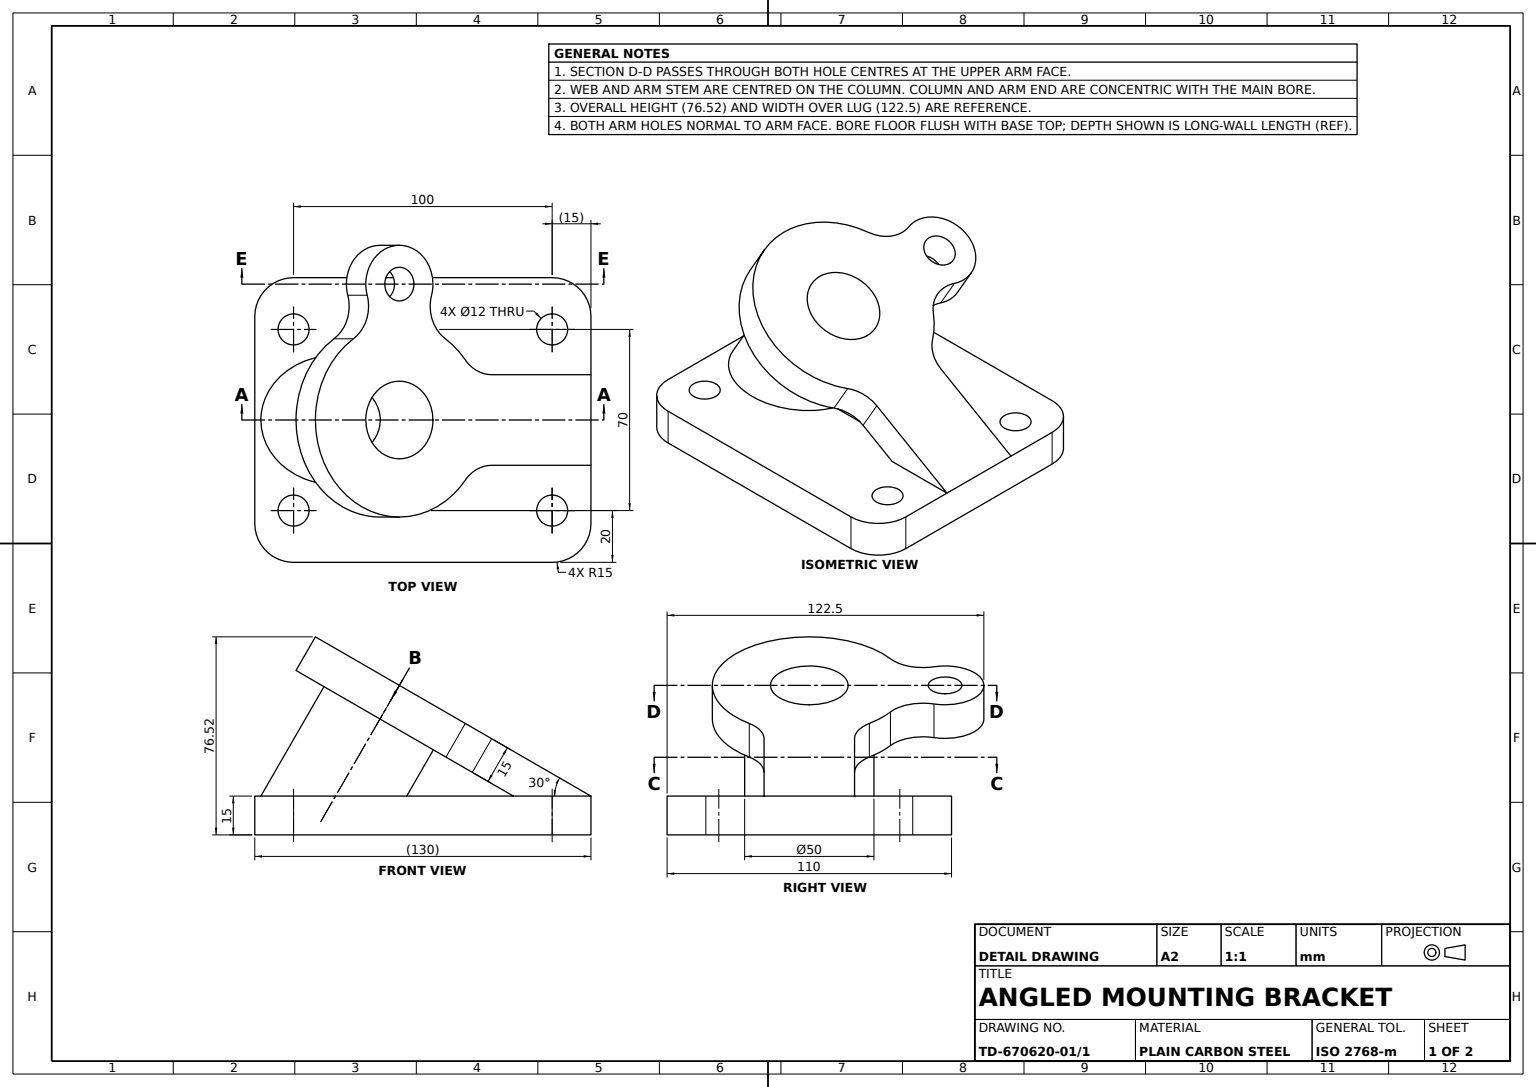
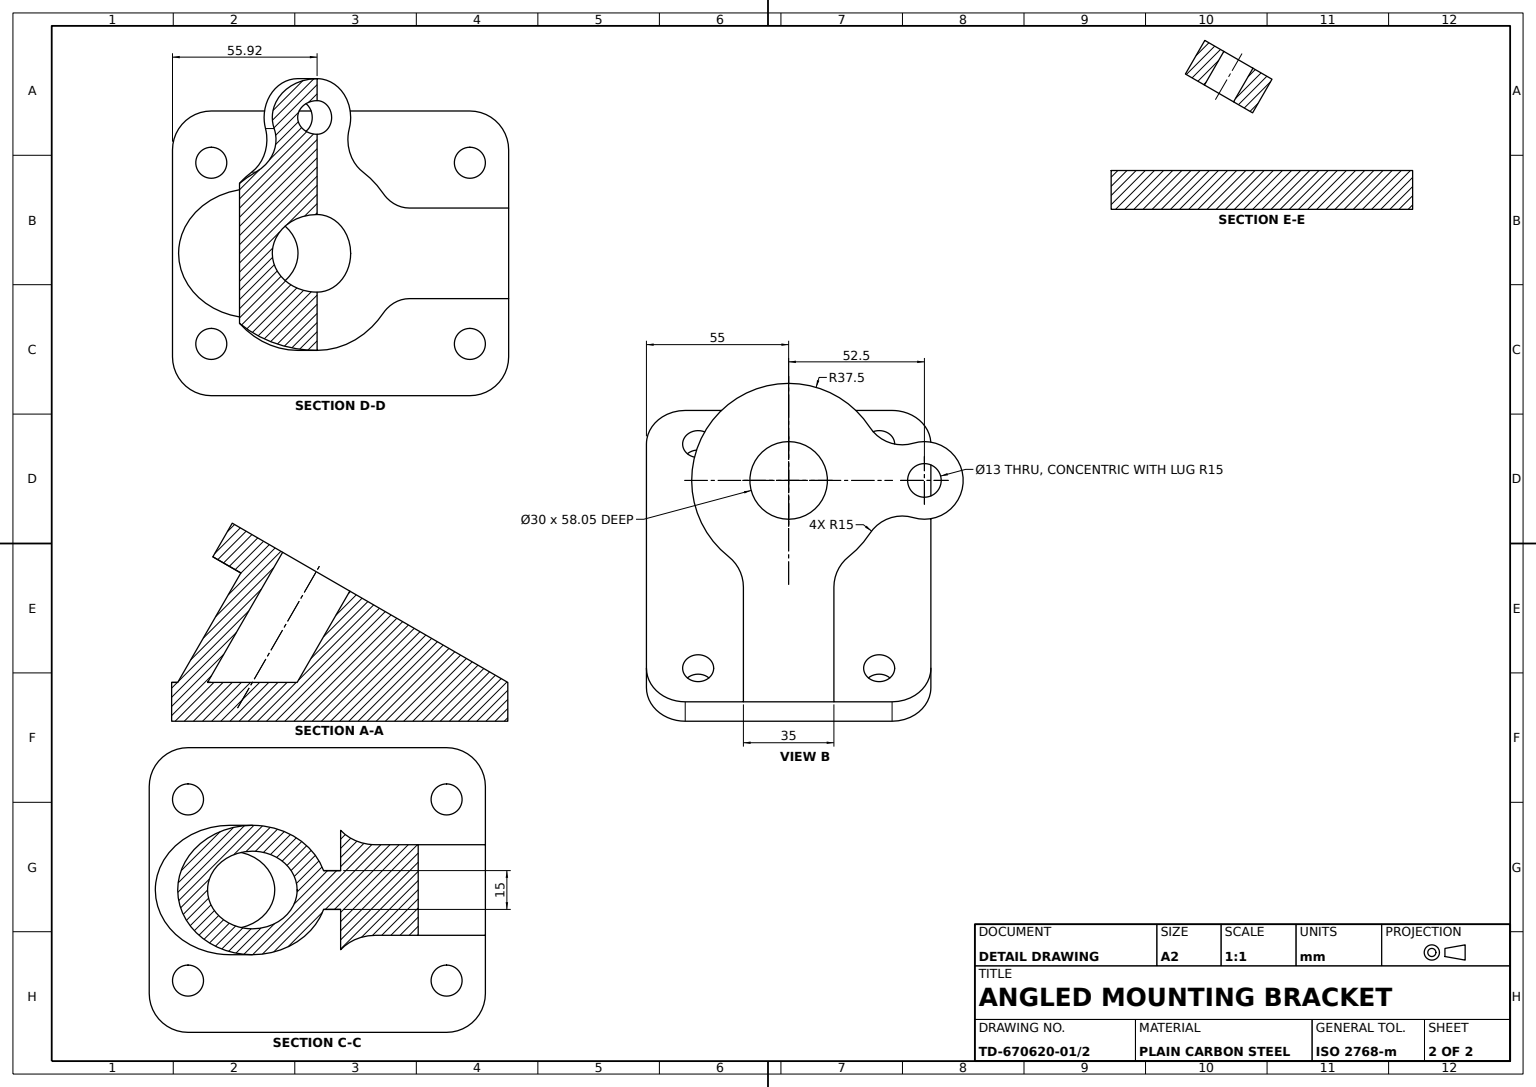
SolidWorks part; units mm, degrees
material "Plain Carbon Steel"
ref_plane "Front Plane" through (0, 0, 0) normal (0, 0, 1) x (1, 0, 0)
ref_plane "Top Plane" through (0, 0, 0) normal (0, 1, 0) x (1, 0, 0)
ref_plane "Right Plane" through (0, 0, 0) normal (1, 0, 0) x (0, 0, -1)
sketch "Base Plate Sketch" plane through (0, 0, 0) normal (0, 1, 0) x (1, 0, 0)
  line L0 (0, 119.1376) -> (0, -127.5955) construction
  line L1 (-50, 55) -> (50, 55)
  line L2 (-65, 40) -> (-65, -40)
  line L3 (-50, -55) -> (50, -55)
  line L4 (65, 40) -> (65, -40)
  line L5 (-65, 55) -> (65, -55) construction
  line L6 (-65, -55) -> (65, 55) construction
  line L7 (107.3268, 0) -> (-125.8206, 0) construction
  circle A0 centre (-50, 35) radius 6
  circle A1 centre (-50, -35) radius 6
  circle A2 centre (50, -35) radius 6
  circle A3 centre (50, 35) radius 6
  arc A4 (50, -55) -> (65, -40) centre (50, -40) ccw
  arc A5 (-65, -40) -> (-50, -55) centre (-50, -40) ccw
  arc A6 (-50, 55) -> (-65, 40) centre (-50, 40) ccw
  arc A7 (50, 55) -> (65, 40) centre (50, 40) cw
  point P0 (0, 0)
  dimension "D8" = 15
  dimension "D9" = 12
  dimension "D10" = 12
  dimension "D11" = 12
  dimension "D1" = 110
  dimension "D2" = 130
  dimension "D3" = 70
  dimension "D4" = 15
  dimension "D5" = 15
  dimension "D6" = 20
  dimension "D7" = 20
  dimension "D12" = 20
  dimension "D13" = 70
extrude "Base Plate" add sketch "Base Plate Sketch" along normal blind 15
sketch "Arm Angle 30deg Layout" plane through (0, 0, 0) normal (0, 0, 1) x (1, 0, 0)
  line L0 (65, 15) -> (-14.8861, 61.1222) construction
  line L1 (-36.1398, 40.7303) -> (56.6599, 40.7303) construction
  dimension "D1" = 30
  dimension "D2" = 92.7997
  dimension "D3" = 36.1398
  dimension "D4" = 40.7303
ref_plane "Plane2" through (22.7452, 39.3958, 0) normal (0.5, 0.866, 0) x (-0.866, 0.5, 0)
sketch "Inclined Arm Sketch" plane through (22.7452, 39.3958, 0) normal (0.5, 0.866, 0) x (-0.866, 0.5, 0)
  line L0 (51.6631, 0) -> (-28.7038, 0) construction
  line L1 (-48.7917, 40) -> (-48.7917, -40) construction
  line L2 (-4.4769, 17.5) -> (-48.7917, 17.5)
  line L5 (-48.7917, 17.5) -> (-48.7917, -17.5)
  line L6 (-48.7917, 0) -> (43.4528, 0) construction
  line L10 (-4.4769, -17.5) -> (-48.7917, -17.5)
  circle A0 centre (36.7542, 0) radius 15
  arc A2 (22.3795, -48.2143) -> (51.1289, -48.2143) centre (36.7542, -52.5) ccw
  arc A3 (57.2895, -31.3776) -> (7.3034, 23.2143) centre (36.7542, 0) ccw
  circle A4 centre (36.7542, -52.5) radius 6.5
  arc A5 (22.3795, -48.2143) -> (16.2189, -31.3776) centre (8.0047, -43.9286) ccw
  arc A6 (57.2895, -31.3776) -> (51.1289, -48.2143) centre (65.5036, -43.9286) ccw
  arc A7 (7.3034, -23.2143) -> (16.2189, -31.3776) centre (36.7542, 0) ccw
  arc A8 (-4.4769, -17.5) -> (7.3034, -23.2143) centre (-4.4769, -32.5) cw
  arc A9 (-4.4769, 17.5) -> (7.3034, 23.2143) centre (-4.4769, 32.5) ccw
  point P23 (3.5879, -17.5)
  dimension "D1" = 30
  dimension "D2" = 36.7542
  dimension "D3" = 30
  dimension "D4" = 75
  dimension "D5" = 13
  dimension "D8" = 30
  dimension "D9" = 30
  dimension "D10" = 15
  dimension "D6" = 35
  dimension "D7" = 17.5
extrude "Inclined Arm" add sketch "Inclined Arm Sketch" against normal blind 15 separate body
sketch "Lug Sketch" plane through (15.2452, 26.4054, 0) normal (-0.5, -0.866, 0) x (0.866, -0.5, 0)
  line L0 (-51.6631, 0) -> (28.7038, 0) construction
  line L1 (-12.9057, -7.5) -> (48.7917, -7.5)
  line L3 (4.4769, -17.5) -> (48.7917, -17.5)
  line L4 (48.7917, -17.5) -> (48.7917, 17.5)
  line L5 (48.7917, 17.5) -> (4.4769, 17.5)
  line L6 (4.4769, -17.5) -> (48.7917, -17.5)
  line L7 (48.7917, -17.5) -> (48.7917, 17.5)
  line L8 (48.7917, 17.5) -> (4.4769, 17.5)
  line L9 (-12.9057, 7.5) -> (48.7917, 7.5)
  line L10 (48.7917, -7.5) -> (48.7917, 7.5)
  line L11 (-11.7542, -7.5) -> (48.7917, 7.5) construction
  line L12 (-11.7542, 7.5) -> (48.7917, -7.5) construction
  circle A0 centre (-36.7542, 0) radius 15 construction
  circle A1 centre (-36.7542, 0) radius 15
  arc A2 (-12.9057, 7.5) -> (-12.9057, -7.5) centre (-36.7542, 0) ccw
  arc A7 (-7.3034, 23.2143) -> (4.4769, 17.5) centre (4.4769, 32.5) ccw
  arc A8 (-7.3034, 23.2143) -> (-57.2895, -31.3776) centre (-36.7542, 0) ccw
  arc A9 (-51.1289, -48.2143) -> (-57.2895, -31.3776) centre (-65.5036, -43.9286) ccw
  arc A10 (-51.1289, -48.2143) -> (-22.3795, -48.2143) centre (-36.7542, -52.5) ccw
  arc A11 (-16.2189, -31.3776) -> (-22.3795, -48.2143) centre (-8.0047, -43.9286) ccw
  arc A12 (-16.2189, -31.3776) -> (-7.3034, -23.2143) centre (-36.7542, 0) ccw
  arc A13 (4.4769, -17.5) -> (-7.3034, -23.2143) centre (4.4769, -32.5) ccw
  arc A14 (-7.3034, 23.2143) -> (4.4769, 17.5) centre (4.4769, 32.5) ccw
  arc A15 (-7.3034, 23.2143) -> (-57.2895, -31.3776) centre (-36.7542, 0) ccw
  arc A16 (-51.1289, -48.2143) -> (-57.2895, -31.3776) centre (-65.5036, -43.9286) ccw
  arc A17 (-51.1289, -48.2143) -> (-22.3795, -48.2143) centre (-36.7542, -52.5) ccw
  arc A18 (-16.2189, -31.3776) -> (-22.3795, -48.2143) centre (-8.0047, -43.9286) ccw
  arc A19 (-16.2189, -31.3776) -> (-7.3034, -23.2143) centre (-36.7542, 0) ccw
  arc A20 (4.4769, -17.5) -> (-7.3034, -23.2143) centre (4.4769, -32.5) ccw
  point P9 (18.5187, 0)
  line M19 (48.7917, -17.5) -> (48.7917, 17.5)
  circle M23 centre (-36.7542, 0) radius 15
  dimension "D2" = 50
  dimension "D3" = 15
  dimension "D4" = 45.5353
  dimension "D1" = 0
extrude "Lug with Bore" add sketch "Lug Sketch" along normal up to body contours L9 A2 L1 M19 M23
